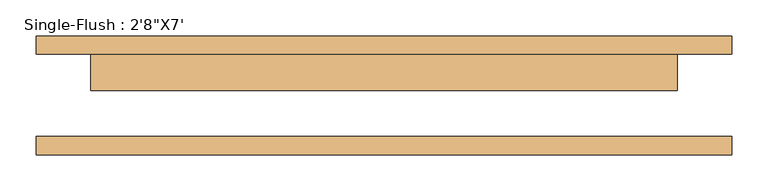
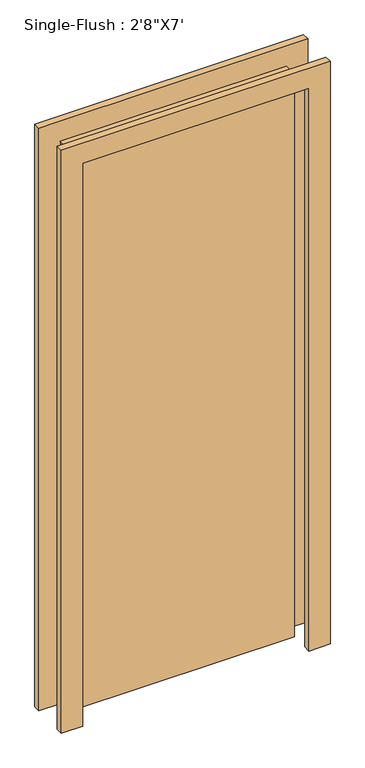
"""IFC4 building model written with IfcOpenShell, lengths in millimetres: door geometry."""

from ifc_helpers import new_model, si_unit, frame, origin, origin_with_axes, place, context, project, spatial, polyline, outline, extrude, source, transform, mapped, element, save


def door_d141acb4(model_context):
    return source(origin(), model_context, "Body", "SweptSolid", [
        extrude(outline(polyline([(2209.8, -482.6), (0.0, -482.6), (0.0, -406.4), (2133.6, -406.4), (2133.6, 406.4), (0.0, 406.4), (0.0, 482.6), (2209.8, 482.6), (2209.8, -482.6)])), frame((0.0, 57.15, 0.0), z_axis=(0.0, 1.0, 0.0), x_axis=(0.0, 0.0, 1.0)), (0.0, 0.0, 1.0), 25.4),
        extrude(outline(polyline([(2209.8, 482.6), (2209.8, -482.6), (0.0, -482.6), (0.0, -406.4), (2133.6, -406.4), (2133.6, 406.4), (0.0, 406.4), (0.0, 482.6), (2209.8, 482.6)])), frame((0.0, -82.55, 0.0), z_axis=(0.0, 1.0, 0.0), x_axis=(0.0, 0.0, 1.0)), (0.0, 0.0, 1.0), 25.4),
        extrude(outline(polyline([(406.4, 6.35), (-406.4, 6.35), (-406.4, 57.15), (406.4, 57.15), (406.4, 6.35)])), origin_with_axes(), (0.0, 0.0, 1.0), 2133.6),
    ])


if __name__ == "__main__":
    model = new_model("IFC4")
    model_context = context("Model", 3, world=origin())
    ifc_project = project(units=[si_unit("LENGTHUNIT", "METRE", prefix="MILLI")], contexts=[model_context])
    site = spatial("IfcSite", under=ifc_project)
    building = spatial("IfcBuilding", under=site)
    placement = place(None, origin())
    door_shape = door_d141acb4(model_context)
    element("IfcDoor", 1, ObjectType="Single-Flush : 2'8\"X7'", at=placement, inside=building, context=model_context, shape_type="MappedRepresentation", body=[
        mapped(door_shape, transform((0.0, 0.0, 0.0), x_axis=(1.0, 0.0, 0.0), y_axis=(0.0, 1.0, 0.0), z_axis=(0.0, 0.0, 1.0))),
    ])
    save(model, "model.ifc")

# Revit data of these elements
# Type "Single-Flush : 2'8\"X7'"
#   Type Mark = "9"
#   Construction Type Id = "MDOOR"
#   Assembly Code = "C1020"
#   Analytic Construction = "Metal"
#   Thickness = 0' - 2"
#   Heat Transfer Coefficient (U) = 0.651978 BTU/(h·ft²·°F)
#   Height = 7' - 0"
#   Trim Projection Ext = 0' - 1"
#   Trim Projection Int = 0' - 1"
#   Trim Width = 0' - 3"
#   Width = 2' - 8"
#   Define Thermal Properties by = 1
#   Door Material = Door - Panel
#   Frame Material = Door - Frame
#   Visual Light Transmittance = 0
#   Solar Heat Gain Coefficient = 0
#   Function = (empty or 0)
#   Wall Closure = (empty or 0)
# Element 1 (IfcDoor, "Single-Flush : 2'8\"X7'")
#   Materials on its faces: "Door - Frame", "Door - Panel"
# Materials
#   "Door - Panel": class "Wood", colour RGB 210 159 95, transparency 0, Cost = 0
#   "Door - Frame": colour RGB 118 70 51, transparency 0, Cost = 0
